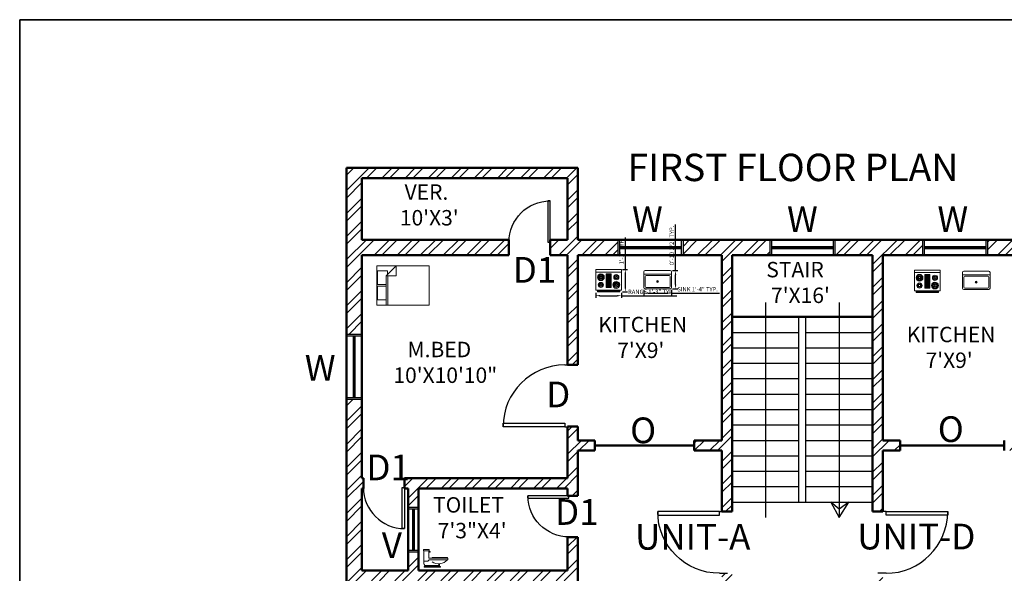
# Model space of a CAD drawing. Units: inches. Extents: x -31842 to -29388, y 18869 to 19743.
# Tile 3 of 12: x -31842 to -31268, y 19420 to 19743. Entities that reach past the tile are written whole.
import ezdxf

# ---------------------------------------------------------------- set-up
doc = ezdxf.new("R2010")
doc.units = ezdxf.units.IN
for name, color, linetype, lineweight in [('A-ANNO-DIMS', 2, 'Continuous', 18), ('A-ANNO-SYMB', 2, 'Continuous', 18), ('A-ANNO-TEXT', 7, 'Continuous', 25), ('A-ANNO-TTLB', 7, 'Continuous', 35), ('A-AREA-IDEN', 3, 'Continuous', 18), ('A-DOOR', 3, 'Continuous', 25), ('A-FLOR-FIXT', 8, 'Continuous', 18), ('A-FLOR-STRS', 7, 'Continuous', 25), ('A-FURN', 8, 'Continuous', 18), ('A-GLAZ', 4, 'Continuous', 25), ('A-WALL', 7, 'Continuous', 50), ('A-WALL-PATT', 8, 'Continuous', 13)]:
    doc.layers.add(name, color=color, linetype=linetype, lineweight=lineweight)
doc.styles.get("Standard").update_dxf_attribs({"font": 'arial.ttf'})
doc.dimstyles.new('ISO-25', dxfattribs={"dimtxt": 2.5, "dimasz": 2.5, "dimexe": 1.25, "dimexo": 0.625, "dimtad": 1, "dimdec": 0, "dimlunit": 3, "dimtxsty": 'Standard', "dimcen": 2.5, "dimadec": 0, "dimazin": 0, "dimtfac": 1, "dimtdec": 0, "dimtmove": 0, "dimatfit": 3, "dimfxl": 1, "dimarcsym": 0})

# ---------------------------------------------------------------- blocks, each defined once
blk = doc.blocks.new('*U8')
for p, q in [((0, 0), (0, -100)), ((750, 0), (750, -100))]:
    blk.add_line(p, q)
blk.add_lwpolyline([(0, 0), (0, 750), (43.75, 750), (43.75, 0)], close=True)
blk.add_arc((0, 0), 750, 0, 90)
blk = doc.blocks.new('Bed - Queen')
for p, q in [((0, -80.00003), (0, 0)), ((0, 0), (59.99999, 0)), ((59.99999, 0), (59.99999, -80.00003)), ((0, -14.4), (44.8, -14.4)), ((7.99999, -1.2), (28.79998, -1.2)), ((7.99999, -14.4), (7.99999, -1.2)), ((28.79998, -1.2), (28.79998, -14.4)), ((31.19999, -1.2), (51.99999, -1.2)), ((31.19999, -14.4), (31.19999, -1.2)), ((59.99999, -29.6), (44.8, -14.4)), ((44.8, -14.4), (44.8, -29.6)), ((51.99999, -1.2), (51.99999, -16.4)), ((44.8, -16.8), (0, -16.8)), ((44.8, -29.6), (59.99999, -29.6)), ((51.99999, -16.4), (46.79936, -16.4)), ((59.99999, -80.00003), (0, -80.00003))]:
    blk.add_line(p, q)
blk = doc.blocks.new('Toilet - side')
for p, q in [((0.5, 5), (0.5, 22)), ((7.5, 22), (7.5, 12)), ((7.5, 21), (9, 21)), ((9, 20), (7.5, 20)), ((9, 21), (9, 20)), ((6, 8), (0.5, 8)), ((22, 2), (2, 2)), ((2, 2), (2, 1)), ((8, 10), (6, 8)), ((7.5, 12), (33, 12)), ((33, 10), (8, 10)), ((32.5, 13), (12, 13)), ((12, 13), (12, 12)), ((21, 4.5), (21, 2)), ((22, 2), (22, 4.5)), ((22, 1), (22, 2)), ((32.5, 12), (32.5, 13)), ((33, 12), (33, 10))]:
    blk.add_line(p, q)
for points in [[(0, 22), (0, 24), (8, 24), (8, 22)], [(1, 0), (1, 1), (23, 1), (23, 0)]]:
    blk.add_lwpolyline(points, close=True)
for centre, radius, start, end in [((3.8, 4.8), 3.26, 175.6013, 237.5288), ((20.3, 20.7), 16.2, 238.1872, 318.7702)]:
    blk.add_arc(centre, radius, start, end)
blk = doc.blocks.new('Range-Oven - 30 in top')
for p, q in [((0, -3), (30, -3)), ((12, -6), (18, -6)), ((13, -20), (13, -6)), ((14, -6), (14, -20)), ((15, -20), (15, -6)), ((16, -6), (16, -20)), ((17, -20), (17, -6)), ((18, -20), (12, -20)), ((6, -24), (6, -25)), ((8, -25), (8, -24)), ((22, -25), (22, -24)), ((24, -24), (24, -25))]:
    blk.add_line(p, q)
for points in [[(0, -24), (0, 0), (30, 0), (30, -24)], [(12, -21), (12, -5), (18, -5), (18, -21)], [(2, -26), (2, -25), (28, -25), (28, -26)]]:
    blk.add_lwpolyline(points, close=True)
for centre, radius in [((6, -9), 4), ((6, -9), 3), ((6, -9), 2), ((6, -9), 1), ((24, -9), 3), ((24, -9), 2), ((24, -9), 1), ((6, -18), 3), ((6, -18), 2), ((6, -18), 1), ((24, -18), 4), ((24, -18), 3), ((24, -18), 2), ((24, -18), 1)]:
    blk.add_circle(centre, radius)
blk = doc.blocks.new('Sink-single - 30 in top')
blk.add_line((-15, -3.999996), (15, -3.999996))
for points in [[(-13.5, 0), (13.5, 0)], [(-15, -18.499996), (-15, -1.5)], [(-13.5, -17.499996), (-13.5, -6.499996)], [(-12.5, -5.499996), (12.5, -5.499996)], [(13.5, -6.499996), (13.5, -17.499996)], [(15, -1.5), (15, -18.499996)], [(13.5, -19.999996), (-13.5, -19.999996)], [(12.5, -18.499996), (-12.5, -18.499996)]]:
    blk.add_lwpolyline(points)
for radius in [1, 0.5]:
    blk.add_circle((0, -11.999996), radius)
for centre, radius, start, end in [((-13.5, -1.5), 1.5, 90, 180), ((-12.5, -6.499996), 1, 90, 180), ((12.5, -6.499996), 1, 0, 90), ((13.5, -1.5), 1.5, 0, 90), ((-13.5, -18.499996), 1.5, 180, 270), ((-12.5, -17.499996), 1, 180, 270), ((12.5, -17.499996), 1, 270, 0), ((13.5, -18.499996), 1.5, 270, 0)]:
    blk.add_arc(centre, radius, start, end)
blk = doc.blocks.new('WIN-3FT')
for p, q in [((0, 36), (9, 36)), ((4, 0), (4, 36)), ((4.5, 0), (4.5, 36)), ((5, 0), (5, 36)), ((0, 0), (9, 0))]:
    blk.add_line(p, q)
blk = doc.blocks.new('*D231')
at = {"layer": 'A-ANNO-DIMS', "color": 0, "lineweight": -2, "transparency": 16777216}
for p, q in [((-31506.05, 19583.98), (-31506.05, 19581.1)), ((-31503.55, 19582.35), (-31493.52, 19582.35)), ((-31491.02, 19583.98), (-31491.02, 19581.1)), ((-31491.02, 19582.35), (-31458.77, 19582.35))]:
    blk.add_line(p, q, dxfattribs=at)
at = {"layer": 'A-ANNO-DIMS', "color": 0, "transparency": 16777216}
for points in [[(-31503.55, 19582.77), (-31503.55, 19581.94), (-31506.05, 19582.35)], [(-31493.52, 19582.77), (-31493.52, 19581.94), (-31491.02, 19582.35)]]:
    blk.add_solid(points, dxfattribs=at)
at = {"layer": 'Defpoints', "color": 0, "transparency": 16777216}
for p in [(-31506.05, 19584.61), (-31491.02, 19584.61), (-31491.02, 19582.35)]:
    blk.add_point(p, dxfattribs=at)
at = {"layer": 'A-ANNO-DIMS', "color": 0, "transparency": 16777216, "insert": (-31473.64, 19584.27), "char_height": 2.5, "attachment_point": 5}
blk.add_mtext('RANGE 1\'-3" TYP.', dxfattribs=at)
blk = doc.blocks.new('*D232')
at = {"layer": 'A-ANNO-DIMS', "color": 0, "lineweight": -2, "transparency": 16777216}
for p, q in [((-31488.76, 19597.64), (-31488.76, 19616.39)), ((-31490.39, 19597.64), (-31487.51, 19597.64)), ((-31488.76, 19587.11), (-31488.76, 19595.14)), ((-31490.39, 19584.61), (-31487.51, 19584.61))]:
    blk.add_line(p, q, dxfattribs=at)
at = {"layer": 'A-ANNO-DIMS', "color": 0, "transparency": 16777216}
for points in [[(-31489.18, 19595.14), (-31488.35, 19595.14), (-31488.76, 19597.64)], [(-31489.18, 19587.11), (-31488.35, 19587.11), (-31488.76, 19584.61)]]:
    blk.add_solid(points, dxfattribs=at)
at = {"layer": 'Defpoints', "color": 0, "transparency": 16777216}
for p in [(-31491.02, 19597.64), (-31488.76, 19597.64), (-31491.02, 19584.61)]:
    blk.add_point(p, dxfattribs=at)
at = {"layer": 'A-ANNO-DIMS', "color": 0, "transparency": 16777216, "insert": (-31490.64, 19608.26), "char_height": 2.5, "attachment_point": 5, "rotation": 90}
blk.add_mtext('1\'-1" TYP.', dxfattribs=at)
blk = doc.blocks.new('*D237')
at = {"layer": 'A-ANNO-DIMS', "color": 0, "lineweight": -2, "transparency": 16777216}
for p, q in [((-31478, 19585.68), (-31478, 19582.64)), ((-31475.5, 19583.89), (-31464.38, 19583.89)), ((-31461.88, 19585.68), (-31461.88, 19582.64)), ((-31461.88, 19583.89), (-31433.78, 19583.89))]:
    blk.add_line(p, q, dxfattribs=at)
at = {"layer": 'A-ANNO-DIMS', "color": 0, "transparency": 16777216}
for points in [[(-31475.5, 19584.3), (-31475.5, 19583.47), (-31478, 19583.89)], [(-31464.38, 19584.3), (-31464.38, 19583.47), (-31461.88, 19583.89)]]:
    blk.add_solid(points, dxfattribs=at)
at = {"layer": 'Defpoints', "color": 0, "transparency": 16777216}
for p in [(-31478, 19586.31), (-31461.88, 19586.31), (-31461.88, 19583.89)]:
    blk.add_point(p, dxfattribs=at)
at = {"layer": 'A-ANNO-DIMS', "color": 0, "transparency": 16777216, "insert": (-31446.58, 19585.8), "char_height": 2.5, "attachment_point": 5}
blk.add_mtext('SINK 1\'-4" TYP.', dxfattribs=at)
blk = doc.blocks.new('*D238')
at = {"layer": 'A-ANNO-DIMS', "color": 0, "lineweight": -2, "transparency": 16777216}
for p, q in [((-31459.46, 19597.05), (-31459.46, 19623.81)), ((-31461.25, 19597.05), (-31458.21, 19597.05)), ((-31459.46, 19588.81), (-31459.46, 19594.55)), ((-31461.25, 19586.31), (-31458.21, 19586.31))]:
    blk.add_line(p, q, dxfattribs=at)
at = {"layer": 'A-ANNO-DIMS', "color": 0, "transparency": 16777216}
for points in [[(-31459.87, 19594.55), (-31459.04, 19594.55), (-31459.46, 19597.05)], [(-31459.87, 19588.81), (-31459.04, 19588.81), (-31459.46, 19586.31)]]:
    blk.add_solid(points, dxfattribs=at)
at = {"layer": 'Defpoints', "color": 0, "transparency": 16777216}
for p in [(-31461.88, 19597.05), (-31459.46, 19597.05), (-31461.88, 19586.31)]:
    blk.add_point(p, dxfattribs=at)
at = {"layer": 'A-ANNO-DIMS', "color": 0, "transparency": 16777216, "insert": (-31461.38, 19611.68), "char_height": 2.5, "attachment_point": 5, "rotation": 90}
blk.add_mtext('0\'-10 1/2" TYP.', dxfattribs=at)

msp = doc.modelspace()

# ---------------------------------------------------------------- hatches: boundary and pattern name
at = {"layer": 'A-WALL-PATT'}
h = msp.add_hatch(dxfattribs=at)
h.set_pattern_fill('ANSI32', color=256)
h.paths.add_polyline_path([(-31119.45, 19656.96), (-31254.45, 19656.96), (-31254.45, 19614.96), (-31277.45, 19614.96), (-31277.45, 19605.96), (-31254.45, 19605.96), (-31254.45, 19555.2), (-31248.45, 19555.2), (-31248.45, 19605.96), (-31240.75, 19605.96), (-31240.75, 19614.96), (-31248.45, 19614.96), (-31248.45, 19650.96), (-31128.45, 19650.96), (-31128.45, 19614.96), (-31216.75, 19614.96), (-31216.75, 19605.96), (-31128.45, 19605.96), (-31128.45, 19559.96), (-31119.45, 19559.96)])
h.paths.add_polyline_path([(-31153.94, 19473.06), (-31153.92, 19475.96), (-31248.45, 19475.96), (-31248.45, 19519.2), (-31251.45, 19519.2), (-31254.45, 19519.2), (-31254.45, 19497.96), (-31267.62, 19497.96), (-31267.62, 19491.96), (-31254.45, 19491.96), (-31254.45, 19465.12), (-31248.45, 19465.12), (-31248.45, 19469.96), (-31161.45, 19469.96), (-31161.45, 19458.96), (-31155.45, 19458.96), (-31155.45, 19469.96), (-31153.94, 19469.96)])
h.paths.add_polyline_path([(-31119.45, 19521.96), (-31128.45, 19521.96), (-31128.45, 19475.96), (-31129.92, 19475.96), (-31129.92, 19469.96), (-31128.45, 19469.96), (-31128.45, 19421.96), (-31155.45, 19421.96), (-31155.45, 19432.96), (-31161.45, 19432.96), (-31161.45, 19421.96), (-31248.45, 19421.96), (-31248.45, 19441.12), (-31254.45, 19441.12), (-31254.45, 19406.17), (-31248.45, 19406.17), (-31248.45, 19415.96), (-31128.45, 19415.96), (-31128.45, 19375.96), (-31119.45, 19375.96)])
h.paths.add_polyline_path([(-31315.45, 19614.96), (-31366.45, 19614.96), (-31366.45, 19605.96), (-31344.45, 19605.96), (-31344.45, 19456.39), (-31338.45, 19456.39), (-31338.45, 19491.96), (-31328.43, 19491.96), (-31328.43, 19497.96), (-31338.45, 19497.96), (-31338.45, 19605.96), (-31315.45, 19605.96)])
h.paths.add_polyline_path([(-31404.45, 19614.96), (-31455.1, 19614.96), (-31455.1, 19605.96), (-31432.45, 19605.96), (-31432.45, 19497.96), (-31448.67, 19497.96), (-31448.67, 19491.96), (-31432.45, 19491.96), (-31432.45, 19456.39), (-31429.07, 19456.39), (-31426.45, 19456.39), (-31426.45, 19605.96), (-31404.45, 19605.96)])
h.paths.add_polyline_path([(-31493.1, 19614.96), (-31516.45, 19614.96), (-31516.45, 19656.96), (-31651.45, 19656.96), (-31651.45, 19559.96), (-31642.45, 19559.96), (-31642.45, 19605.96), (-31556.65, 19605.96), (-31556.65, 19614.96), (-31642.45, 19614.96), (-31642.45, 19650.96), (-31522.45, 19650.96), (-31522.45, 19614.96), (-31532.65, 19614.96), (-31532.65, 19613.66), (-31532.65, 19610.46), (-31532.65, 19605.96), (-31522.45, 19605.96), (-31522.45, 19541.95), (-31516.45, 19541.95), (-31516.45, 19605.96), (-31493.1, 19605.96)])
h.paths.add_polyline_path([(-31642.45, 19521.96), (-31651.45, 19521.96), (-31651.45, 19374.96), (-31642.45, 19374.96), (-31642.45, 19415.96), (-31522.45, 19415.96), (-31522.45, 19406.54), (-31516.45, 19406.54), (-31516.45, 19441.56), (-31522.45, 19441.56), (-31522.45, 19421.96), (-31609.45, 19421.96), (-31609.45, 19432.96), (-31615.45, 19432.96), (-31615.45, 19421.96), (-31642.45, 19421.96), (-31642.45, 19469.96), (-31641.6, 19469.96), (-31641.6, 19475.96), (-31642.45, 19475.96)])
h.paths.add_polyline_path([(-31516.45, 19491.96), (-31506.54, 19491.96), (-31506.54, 19497.96), (-31516.45, 19497.96), (-31516.45, 19505.95), (-31522.45, 19505.95), (-31522.45, 19475.96), (-31617.6, 19475.96), (-31617.6, 19469.96), (-31615.45, 19469.96), (-31615.45, 19458.96), (-31609.45, 19458.96), (-31609.45, 19469.96), (-31522.45, 19469.96), (-31522.45, 19465.56), (-31516.45, 19465.56)])
h.paths.add_polyline_path([(-31248.45, 19370.17), (-31251.45, 19370.17), (-31254.45, 19370.17), (-31254.45, 19297.96), (-31338.45, 19297.96), (-31338.45, 19420.39), (-31344.45, 19420.39), (-31344.45, 19413.96), (-31346.02, 19413.96), (-31346.02, 19407.96), (-31344.45, 19407.96), (-31344.45, 19291.96), (-31213.45, 19291.96), (-31213.45, 19275.43), (-31207.45, 19275.43), (-31207.45, 19291.96), (-31128.45, 19291.96), (-31128.45, 19274.96), (-31119.45, 19274.96), (-31119.45, 19337.96), (-31128.45, 19337.96), (-31128.45, 19297.96), (-31248.45, 19297.96)])
h.paths.add_polyline_path([(-31426.45, 19407.96), (-31424.99, 19407.96), (-31424.99, 19410.83), (-31424.95, 19413.96), (-31426.45, 19413.96), (-31426.45, 19420.39), (-31432.45, 19420.39), (-31432.45, 19295.96), (-31516.45, 19295.96), (-31516.45, 19370.54), (-31522.45, 19370.54), (-31522.45, 19295.96), (-31642.45, 19295.96), (-31642.45, 19336.96), (-31651.45, 19336.96), (-31651.45, 19272.96), (-31642.45, 19272.96), (-31642.45, 19289.96), (-31563.45, 19289.96), (-31563.45, 19270.05), (-31557.45, 19270.05), (-31557.45, 19289.96), (-31426.45, 19289.96)])
h.paths.add_polyline_path([(-31557.45, 19222.83), (-31563.45, 19222.83), (-31563.45, 19217.96), (-31642.45, 19217.96), (-31642.45, 19234.96), (-31651.45, 19234.96), (-31651.45, 19201.96), (-31642.45, 19201.96), (-31642.45, 19211.96), (-31563.45, 19211.96), (-31563.45, 19206.27), (-31562.72, 19206.27), (-31559.53, 19206.27), (-31557.45, 19206.18)])
h.paths.add_polyline_path([(-31553.97, 19163.65), (-31553.95, 19165.96), (-31557.45, 19165.96), (-31557.45, 19182.18), (-31563.45, 19182.18), (-31563.45, 19165.96), (-31639.16, 19165.96), (-31639.16, 19159.96), (-31630.45, 19159.96), (-31630.45, 19110.96), (-31624.45, 19110.96), (-31624.45, 19159.96), (-31553.97, 19159.96)])
h.paths.add_polyline_path([(-31663.16, 19165.96), (-31681.45, 19165.96), (-31681.45, 19014.96), (-31592.45, 19014.96), (-31592.45, 19023.96), (-31624.45, 19023.96), (-31624.45, 19072.96), (-31630.45, 19072.96), (-31630.45, 19023.96), (-31675.45, 19023.96), (-31675.45, 19159.96), (-31663.16, 19159.96)])
h.paths.add_polyline_path([(-31516.45, 19159.96), (-31505.99, 19159.96), (-31505.99, 19165.96), (-31524.95, 19165.96), (-31524.95, 19159.96), (-31522.45, 19159.96), (-31522.45, 19023.96), (-31554.45, 19023.96), (-31554.45, 19014.96), (-31471.45, 19014.96), (-31471.45, 19023.96), (-31516.45, 19023.96)])
h.paths.add_polyline_path([(-31337.45, 19023.96), (-31382.45, 19023.96), (-31382.45, 19159.96), (-31299.75, 19159.96), (-31299.75, 19165.96), (-31344.45, 19165.96), (-31382.45, 19165.96), (-31382.45, 19407.96), (-31382.02, 19413.96), (-31388.95, 19413.96), (-31388.95, 19407.96), (-31388.45, 19407.96), (-31388.45, 19165.96), (-31432.45, 19165.96), (-31469.99, 19165.96), (-31469.99, 19159.96), (-31432.45, 19159.96), (-31388.45, 19159.96), (-31388.45, 19023.96), (-31433.45, 19023.96), (-31433.45, 19014.96), (-31337.45, 19014.96)])
h.paths.add_polyline_path([(-31216.45, 19023.96), (-31248.45, 19023.96), (-31248.45, 19159.96), (-31245.93, 19159.96), (-31245.93, 19162.87), (-31245.93, 19165.96), (-31254.45, 19165.96), (-31263.75, 19165.96), (-31263.75, 19159.96), (-31254.45, 19159.96), (-31254.45, 19023.96), (-31299.45, 19023.96), (-31299.45, 19014.96), (-31216.45, 19014.96)])
h.paths.add_polyline_path([(-31089.45, 19165.96), (-31110.75, 19165.96), (-31110.75, 19159.96), (-31095.45, 19159.96), (-31095.45, 19023.96), (-31140.45, 19023.96), (-31140.45, 19072.96), (-31146.45, 19072.96), (-31146.45, 19023.96), (-31178.45, 19023.96), (-31178.45, 19014.96), (-31089.45, 19014.96)])
h.paths.add_polyline_path([(-31134.75, 19165.96), (-31207.45, 19165.96), (-31207.45, 19182.5), (-31213.45, 19182.5), (-31213.45, 19165.96), (-31216.93, 19165.96), (-31216.93, 19159.96), (-31146.45, 19159.96), (-31146.45, 19110.96), (-31140.45, 19110.96), (-31140.45, 19159.96), (-31134.75, 19159.96)])
h.paths.add_polyline_path([(-31119.45, 19236.96), (-31128.45, 19236.96), (-31128.45, 19219.96), (-31207.45, 19219.96), (-31207.45, 19227.12), (-31213.45, 19227.12), (-31213.45, 19206.5), (-31207.45, 19206.5), (-31207.45, 19213.96), (-31128.45, 19213.96), (-31128.45, 19202.96), (-31119.45, 19202.96)])

# ---------------------------------------------------------------- linework, layer by layer
at = {"layer": 'A-ANNO-TTLB'}
msp.add_lwpolyline([(-31842.18, 19743.36), (-29387.67, 19743.36), (-29387.67, 18868.82), (-31842.18, 18868.82)], close=True, dxfattribs=at)
at = {"layer": 'A-FLOR-STRS'}
for p, q in [((-31406.95, 19578.43), (-31406.95, 19453.01)), ((-31363.95, 19578.43), (-31363.95, 19453.01)), ((-31387.45, 19461.96), (-31387.45, 19569.96)), ((-31383.45, 19461.96), (-31383.45, 19569.96)), ((-31426.45, 19560.96), (-31387.45, 19560.96)), ((-31383.45, 19560.96), (-31344.45, 19560.96)), ((-31426.45, 19551.96), (-31387.45, 19551.96)), ((-31383.45, 19551.96), (-31344.45, 19551.96)), ((-31426.45, 19542.96), (-31387.45, 19542.96)), ((-31383.45, 19542.96), (-31344.45, 19542.96)), ((-31426.45, 19533.96), (-31387.45, 19533.96)), ((-31383.45, 19533.96), (-31344.45, 19533.96)), ((-31426.45, 19524.96), (-31387.45, 19524.96)), ((-31383.45, 19524.96), (-31344.45, 19524.96)), ((-31426.45, 19515.96), (-31387.45, 19515.96)), ((-31383.45, 19515.96), (-31344.45, 19515.96)), ((-31426.45, 19506.96), (-31387.45, 19506.96)), ((-31383.45, 19506.96), (-31344.45, 19506.96)), ((-31426.45, 19497.96), (-31387.45, 19497.96)), ((-31383.45, 19497.96), (-31344.45, 19497.96)), ((-31426.45, 19488.96), (-31387.45, 19488.96)), ((-31383.45, 19488.96), (-31344.45, 19488.96)), ((-31426.45, 19479.96), (-31387.45, 19479.96)), ((-31383.45, 19479.96), (-31344.45, 19479.96)), ((-31426.45, 19470.96), (-31387.45, 19470.96)), ((-31383.45, 19470.96), (-31344.45, 19470.96)), ((-31426.45, 19461.96), (-31344.45, 19461.96)), ((-31363.95, 19457.88), (-31368.8, 19461.96)), ((-31368.8, 19461.96), (-31363.95, 19453.01)), ((-31363.95, 19453.01), (-31358.35, 19461.96)), ((-31358.35, 19461.96), (-31363.95, 19457.88))]:
    msp.add_line(p, q, dxfattribs=at)
at = {"layer": 'A-GLAZ'}
for p, q in [((-31493.1, 19614.96), (-31493.1, 19605.96)), ((-31455.1, 19614.96), (-31455.1, 19605.96)), ((-31404.45, 19614.96), (-31404.45, 19605.96)), ((-31366.45, 19614.96), (-31366.45, 19605.96)), ((-31315.45, 19614.96), (-31315.45, 19605.96)), ((-31277.45, 19614.96), (-31277.45, 19605.96)), ((-31651.45, 19559.96), (-31642.45, 19559.96)), ((-31651.45, 19521.96), (-31642.45, 19521.96)), ((-31615.45, 19458.96), (-31609.45, 19458.96)), ((-31615.45, 19458.96), (-31609.45, 19458.96)), ((-31615.45, 19457.96), (-31609.45, 19457.96)), ((-31615.45, 19457.96), (-31609.45, 19457.96)), ((-31612.95, 19457.96), (-31612.95, 19433.96)), ((-31612.95, 19457.96), (-31612.95, 19433.96)), ((-31612.45, 19457.96), (-31612.45, 19433.96)), ((-31612.45, 19457.96), (-31612.45, 19433.96)), ((-31611.95, 19457.96), (-31611.95, 19433.96)), ((-31611.95, 19457.96), (-31611.95, 19433.96)), ((-31615.45, 19433.96), (-31609.45, 19433.96)), ((-31615.45, 19433.96), (-31609.45, 19433.96)), ((-31615.45, 19432.96), (-31609.45, 19432.96)), ((-31615.45, 19432.96), (-31609.45, 19432.96))]:
    msp.add_line(p, q, dxfattribs=at)
at = {"layer": 'A-WALL'}
for p, q in [((-31651.45, 19165.96), (-31651.45, 19656.96)), ((-31651.45, 19656.96), (-31516.45, 19656.96)), ((-31516.45, 19614.96), (-31516.45, 19656.96)), ((-31642.45, 19650.96), (-31522.45, 19650.96)), ((-31642.45, 19614.96), (-31642.45, 19650.96)), ((-31522.45, 19614.96), (-31522.45, 19650.96)), ((-31642.45, 19614.96), (-31556.65, 19614.96)), ((-31556.65, 19614.96), (-31556.65, 19605.96)), ((-31532.65, 19614.96), (-31532.65, 19605.96)), ((-31532.65, 19614.96), (-31522.45, 19614.96)), ((-31516.45, 19614.96), (-31254.45, 19614.96)), ((-31642.45, 19605.96), (-31556.65, 19605.96)), ((-31642.45, 19475.96), (-31642.45, 19605.96)), ((-31532.65, 19605.96), (-31522.45, 19605.96)), ((-31522.45, 19541.95), (-31522.45, 19605.96)), ((-31516.45, 19605.96), (-31432.45, 19605.96)), ((-31516.45, 19541.95), (-31516.45, 19605.96)), ((-31432.45, 19497.96), (-31432.45, 19605.96)), ((-31426.45, 19605.96), (-31344.45, 19605.96)), ((-31426.45, 19456.39), (-31426.45, 19605.96)), ((-31344.45, 19605.96), (-31344.45, 19456.39)), ((-31338.45, 19605.96), (-31338.45, 19497.96)), ((-31338.45, 19605.96), (-31254.45, 19605.96)), ((-31426.45, 19569.96), (-31344.45, 19569.96)), ((-31522.45, 19541.95), (-31516.45, 19541.95)), ((-31522.45, 19475.96), (-31522.45, 19505.95)), ((-31522.45, 19505.95), (-31516.45, 19505.95)), ((-31516.45, 19497.96), (-31516.45, 19505.95)), ((-31516.45, 19497.96), (-31506.54, 19497.96)), ((-31506.54, 19497.96), (-31506.54, 19491.96)), ((-31506.54, 19494.96), (-31448.67, 19494.96)), ((-31448.67, 19497.96), (-31448.67, 19491.96)), ((-31448.67, 19497.96), (-31432.45, 19497.96)), ((-31338.45, 19497.96), (-31328.43, 19497.96)), ((-31328.43, 19497.96), (-31328.43, 19491.96)), ((-31328.43, 19494.96), (-31267.62, 19494.96)), ((-31267.62, 19497.96), (-31267.62, 19491.96)), ((-31516.45, 19491.96), (-31506.54, 19491.96)), ((-31516.45, 19465.56), (-31516.45, 19491.96)), ((-31448.67, 19491.96), (-31432.45, 19491.96)), ((-31432.45, 19456.39), (-31432.45, 19491.96)), ((-31338.45, 19491.96), (-31338.45, 19456.39)), ((-31338.45, 19491.96), (-31328.43, 19491.96)), ((-31642.45, 19475.96), (-31641.6, 19475.96)), ((-31641.6, 19475.96), (-31641.6, 19469.96)), ((-31617.6, 19475.96), (-31617.6, 19469.96)), ((-31617.6, 19475.96), (-31522.45, 19475.96)), ((-31642.45, 19469.96), (-31641.6, 19469.96)), ((-31642.45, 19421.96), (-31642.45, 19469.96)), ((-31617.6, 19469.96), (-31615.45, 19469.96)), ((-31615.45, 19421.96), (-31615.45, 19469.96)), ((-31609.45, 19469.96), (-31522.45, 19469.96)), ((-31609.45, 19421.96), (-31609.45, 19469.96)), ((-31522.45, 19465.56), (-31522.45, 19469.96)), ((-31522.45, 19465.56), (-31516.45, 19465.56)), ((-31426.45, 19456.39), (-31432.45, 19456.39)), ((-31344.45, 19456.39), (-31338.45, 19456.39)), ((-31522.45, 19421.96), (-31522.45, 19441.56)), ((-31522.45, 19441.56), (-31516.45, 19441.56)), ((-31516.45, 19406.54), (-31516.45, 19441.56)), ((-31642.45, 19421.96), (-31615.45, 19421.96)), ((-31609.45, 19421.96), (-31522.45, 19421.96))]:
    msp.add_line(p, q, dxfattribs=at)

# ---------------------------------------------------------------- block references
at = {"layer": 'A-DOOR', "xscale": -0.0319999993054766, "yscale": 0.0319999993054766, "zscale": 0.0319999993054766}
msp.add_blockref('*U8', (-31532.65, 19613.66), dxfattribs=at)
at = {"layer": 'A-DOOR'}
for p, xscale, yscale, zscale, rotation in [((-31524.06, 19505.93), 0.0480180772456396, 0.0480180772456396, 0.0480180772456396, 90.00000000000003), ((-31617.6, 19470.48), 0.0320000000000009, 0.0320000000000009, 0.0320000000000009, 180), ((-31521.64, 19465.56), -0.0319267259435146, 0.0319267259435146, 0.0319267259435146, 90), ((-31433.87, 19456.39), -0.0480027575407148, 0.0480027575407148, 0.0480027575407148, 90), ((-31336.65, 19456.39), 0.0479999979369979, 0.0479999979369979, 0.0479999979369979, 270)]:
    msp.add_blockref('*U8', p, dxfattribs=dict(at, xscale=xscale, yscale=yscale, zscale=zscale, rotation=rotation))
at = {"layer": 'A-FLOR-FIXT'}
for name, p, xscale, yscale, zscale in [('Range-Oven - 30 in top', (-31506.05, 19597.64), 0.501109879279097, 0.501109879279097, 0.501109879279097), ('Sink-single - 30 in top', (-31469.94, 19597.05), 0.537483841617589, 0.537483841617589, 0.537483841617589), ('Range-Oven - 30 in top', (-31320.1, 19597.3), 0.501109879279097, 0.501109879279097, 0.501109879279097), ('Sink-single - 30 in top', (-31283.99, 19596.72), 0.537483841617589, 0.537483841617589, 0.537483841617589), ('Toilet - side', (-31606.63, 19424), 0.4314503559530352, 0.4314503559530352, 0.4314503559530352)]:
    msp.add_blockref(name, p, dxfattribs=dict(at, xscale=xscale, yscale=yscale, zscale=zscale))
at = {"layer": 'A-FURN', "xscale": 0.382279819255463, "yscale": 0.382279819255463, "zscale": 0.382279819255463, "rotation": 90}
msp.add_blockref('Bed - Queen', (-31633.79, 19576.9), dxfattribs=at)
at = {"layer": 'A-GLAZ'}
for p, rotation in [((-31492.1, 19614.96), 269.9999999999727), ((-31403.45, 19614.96), 269.9999999999837), ((-31314.45, 19614.96), 269.9999999999837)]:
    msp.add_blockref('WIN-3FT', p, dxfattribs=dict(at, rotation=rotation))
msp.add_blockref('WIN-3FT', (-31651.45, 19522.96), dxfattribs=at)

# ---------------------------------------------------------------- texts
at = {"layer": 'A-ANNO-SYMB', "char_height": 15, "attachment_point": 1}
for s, insert in [('{W}', (-31484.87, 19634.55)), ('{W}', (-31394.41, 19634.55)), ('{W}', (-31306.65, 19634.55)), ('{D1}', (-31554.47, 19604.92)), ('{W}', (-31675.81, 19547.75)), ('{D}', (-31534.97, 19532.23)), ('{O}', (-31306.44, 19511.97)), ('{O}', (-31485.96, 19511.29)), ('{D1}', (-31639.88, 19489.66)), ('{D1}', (-31529.8, 19463.65)), ('{V}', (-31630.88, 19444.3))]:
    msp.add_mtext_dynamic_manual_height_columns(s, width=533.5224, gutter_width=12.5, heights=[0], dxfattribs=dict(at, insert=insert))
at = {"layer": 'A-ANNO-TEXT', "insert": (-31487.46, 19665.18), "char_height": 16, "attachment_point": 1}
msp.add_mtext_dynamic_manual_height_columns('{FIRST FLOOR PLAN}', width=477.9643, gutter_width=12.5, heights=[0], dxfattribs=at)
at = {"layer": 'A-AREA-IDEN', "attachment_point": 1}
for s, width, insert, char_height in [("{\\H3.6x;   VER.\\P  10'X3'}", 652.6959, (-31625.83, 19647.31), 2.5), ("{\\H3.6x;   STAIR\\P    7'X16'}", 652.6959, (-31414.75, 19602.06), 2.5), ("{\\H3.6x;  KITCHEN\\P      7'X9'}", 652.6959, (-31510, 19570), 2.5), ("{\\H3.6x;KITCHEN\\P    7'X9'}", 652.6959, (-31324.56, 19564.2), 2.5), ('{\\H3.6x;   M.BED\\P10\'X10\'10"}', 652.6959, (-31624.12, 19555.46), 2.5), ('{\\H3.6x; TOILET\\P  7\'3"X4\'}', 652.6959, (-31603.71, 19464.81), 2.5), ('{UNIT-A}', 533.5224, (-31483.09, 19449.17), 15), ('{UNIT-D}', 533.5224, (-31353.47, 19449.32), 15)]:
    msp.add_mtext_dynamic_manual_height_columns(s, width=width, gutter_width=12.5, heights=[0], dxfattribs=dict(at, insert=insert, char_height=char_height))

# ---------------------------------------------------------------- dimensions: what is measured, and where the dimension line sits
at = {"layer": 'A-ANNO-DIMS'}
for base, p1, p2, picture, middle in [((-31459.46, 19597.05), (-31461.88, 19586.31), (-31461.88, 19597.05), '*D238', (-31461.38, 19611.68)), ((-31488.76, 19597.64), (-31491.02, 19584.61), (-31491.02, 19597.64), '*D232', (-31490.64, 19608.26))]:
    dim = msp.add_linear_dim(base=base, p1=p1, p2=p2, angle=90, text='<> TYP.', dimstyle='ISO-25', override={"dimdec": 1, "dimlfac": 1, "dimrnd": 0, "dimzin": 1, "dimdsep": 46, "dimlunit": 4, "dimfrac": 2}, dxfattribs=at)
    dim.commit()
    dim.dimension.update_dxf_attribs({"geometry": picture, "text_midpoint": middle})
for base, p1, p2, text, picture, middle in [((-31491.02, 19582.35), (-31506.05, 19584.61), (-31491.02, 19584.61), 'RANGE <> TYP.', '*D231', (-31473.64, 19584.27)), ((-31461.88, 19583.89), (-31478, 19586.31), (-31461.88, 19586.31), 'SINK <> TYP.', '*D237', (-31446.58, 19585.8))]:
    dim = msp.add_linear_dim(base=base, p1=p1, p2=p2, text=text, dimstyle='ISO-25', override={"dimdec": 1, "dimlfac": 1, "dimrnd": 0, "dimzin": 1, "dimdsep": 46, "dimlunit": 4, "dimfrac": 2}, dxfattribs=at)
    dim.commit()
    dim.dimension.update_dxf_attribs({"geometry": picture, "text_midpoint": middle})

doc.saveas('drawing.dxf')
